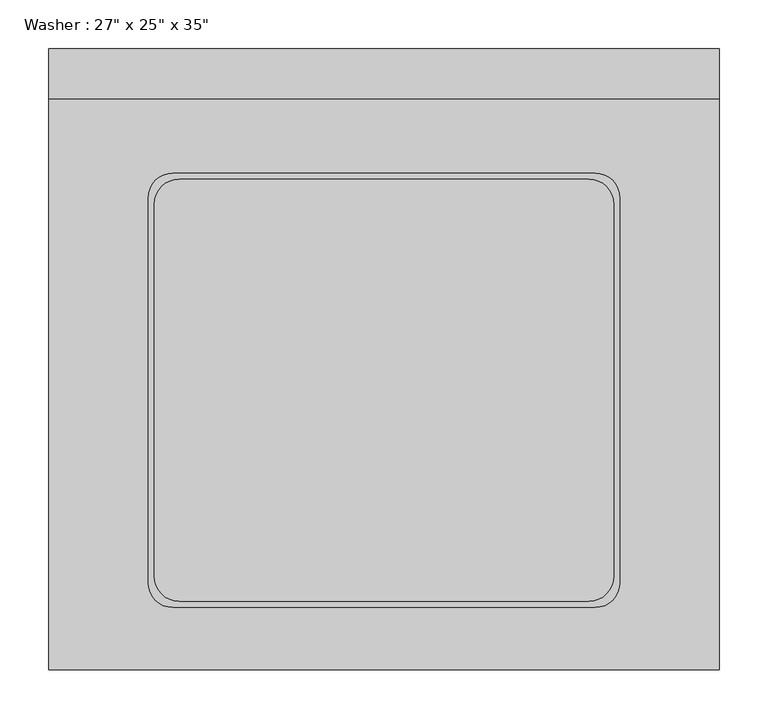
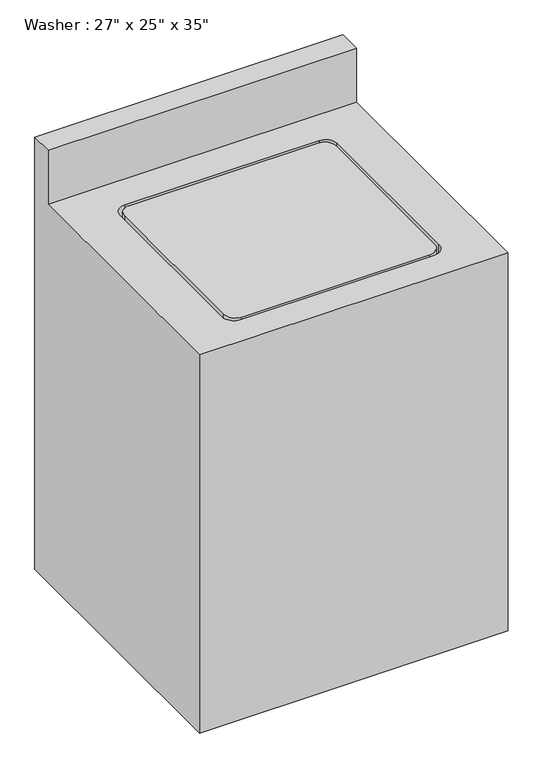
"""IFC4 building model written with IfcOpenShell, lengths in millimetres: proxy geometry."""

from ifc_helpers import new_model, si_unit, point, frame, frame_2d, origin, place, context, project, spatial, polyline, circle_curve, trimmed, segment, composite_curve, outline, extrude, source, transform, mapped, element, save
from ifc_brep_helpers import plane_surface, revolved_surface, advanced_brep


def proxy_e75280ca(model_context):
    return source(origin(), model_context, "Body", "SolidModel", [
        advanced_brep(
        [(77.5174685, 545.8495648, 889.0), (77.5174685, 545.8495648, 1016.0), (77.5174685, 596.6495648, 1016.0), (77.5174685, 596.6495648, 0.0), (77.5174685, -38.3504352, 0.0), (77.5174685, -38.3504352, 889.0), (763.3174685, 596.6495648, 1016.0), (763.3174685, 545.8495648, 1016.0), (763.3174685, 545.8495648, 889.0), (763.3174685, -38.3504352, 889.0), (763.3174685, -38.3504352, 0.0), (763.3174685, 596.6495648, 0.0), (204.5174685, 469.4681955, 889.0), (636.3174685, 469.4681955, 889.0), (661.7174685, 444.0681955, 889.0), (661.7174685, 50.5495648, 889.0), (636.3174685, 25.1495648, 889.0), (204.5174685, 25.1495648, 889.0), (179.1174685, 50.5495648, 889.0), (179.1174685, 444.0681955, 889.0), (636.3174685, 469.4681955, 838.2), (204.5174685, 469.4681955, 838.2), (179.1174685, 444.0681955, 838.2), (179.1174685, 50.5495648, 838.2), (204.5174685, 25.1495648, 838.2), (636.3174685, 25.1495648, 838.2), (661.7174685, 50.5495648, 838.2), (661.7174685, 444.0681955, 838.2)],
        [
            (0, 1),
            (1, 2),
            (2, 3),
            (3, 4),
            (4, 5),
            (5, 0),
            (6, 7),
            (7, 8),
            (8, 9),
            (9, 10),
            (10, 11),
            (11, 6),
            (0, 8),
            (7, 1),
            (6, 2),
            (11, 3),
            (5, 9),
            (12, 13),
            (13, 14, circle_curve(frame((636.3174685, 444.0681955, 889.0), z_axis=(0.0, 0.0, -1.0), x_axis=(0.0, -1.0, 0.0)), 25.4)),
            (14, 15),
            (15, 16, circle_curve(frame((636.3174685, 50.5495648, 889.0), z_axis=(0.0, 0.0, -1.0), x_axis=(0.0, -1.0, 0.0)), 25.4)),
            (16, 17),
            (17, 18, circle_curve(frame((204.5174685, 50.5495648, 889.0), z_axis=(0.0, 0.0, -1.0), x_axis=(0.0, -1.0, 0.0)), 25.4)),
            (18, 19),
            (19, 12, circle_curve(frame((204.5174685, 444.0681955, 889.0), z_axis=(0.0, 0.0, -1.0), x_axis=(0.0, -1.0, 0.0)), 25.4)),
            (10, 4),
            (20, 21),
            (21, 22, circle_curve(frame((204.5174685, 444.0681955, 838.2), z_axis=(0.0, 0.0, 1.0), x_axis=(0.0, -1.0, 0.0)), 25.4)),
            (22, 23),
            (23, 24, circle_curve(frame((204.5174685, 50.5495648, 838.2), z_axis=(0.0, 0.0, 1.0), x_axis=(0.0, -1.0, 0.0)), 25.4)),
            (24, 25),
            (25, 26, circle_curve(frame((636.3174685, 50.5495648, 838.2), z_axis=(0.0, 0.0, 1.0), x_axis=(0.0, -1.0, 0.0)), 25.4)),
            (26, 27),
            (27, 20, circle_curve(frame((636.3174685, 444.0681955, 838.2), z_axis=(0.0, 0.0, 1.0), x_axis=(0.0, -1.0, 0.0)), 25.4)),
            (20, 13),
            (12, 21),
            (19, 22),
            (18, 23),
            (17, 24),
            (16, 25),
            (15, 26),
            (14, 27),
        ],
        [
            plane_surface(frame((77.5174685, 545.8495648, 889.0), z_axis=(-1.0, 0.0, 0.0), x_axis=(0.0, 0.0, 1.0))),
            plane_surface(frame((763.3174685, 545.8495648, 889.0), z_axis=(1.0, 0.0, 0.0), x_axis=(0.0, 0.0, -1.0))),
            plane_surface(frame((77.5174685, 545.8495648, 889.0), z_axis=(0.0, -1.0, 0.0), x_axis=(1.0, 0.0, 0.0))),
            plane_surface(frame((77.5174685, 545.8495648, 1016.0), z_axis=(0.0, 0.0, 1.0), x_axis=(1.0, 0.0, 0.0))),
            plane_surface(frame((77.5174685, 596.6495648, 1016.0), z_axis=(0.0, 1.0, 0.0), x_axis=(1.0, 0.0, 0.0))),
            plane_surface(frame((77.5174685, -38.3504352, 889.0), z_axis=(0.0, 0.0, 1.0), x_axis=(0.0, -1.0, 0.0))),
            plane_surface(frame((77.5174685, -38.3504352, 0.0), z_axis=(0.0, 0.0, -1.0), x_axis=(0.0, 1.0, 0.0))),
            plane_surface(frame((77.5174685, -38.3504352, 889.0), z_axis=(0.0, -1.0, 0.0), x_axis=(0.0, 0.0, -1.0))),
            plane_surface(frame((204.5174685, 469.4681955, 838.2), z_axis=(0.0, 0.0, 1.0), x_axis=(1.0, 0.0, 0.0))),
            plane_surface(frame((636.3174685, 469.4681955, 889.0), z_axis=(0.0, -1.0, 0.0), x_axis=(0.0, 0.0, -1.0))),
            revolved_surface(polyline([(204.5174685, 418.6681955, 889.0), (204.5174685, 418.6681955, 838.2)]), (204.5174685, 444.0681955, 838.2), (0.0, 0.0, 1.0)),
            plane_surface(frame((179.1174685, 444.0681955, 889.0), z_axis=(1.0, 0.0, 0.0), x_axis=(0.0, 0.0, -1.0))),
            revolved_surface(polyline([(204.5174685, 25.1495648, 889.0), (204.5174685, 25.1495648, 838.2)]), (204.5174685, 50.5495648, 838.2), (0.0, 0.0, 1.0)),
            plane_surface(frame((204.5174685, 25.1495648, 889.0), z_axis=(0.0, 1.0, 0.0), x_axis=(0.0, 0.0, -1.0))),
            revolved_surface(polyline([(636.3174685, 25.1495648, 889.0), (636.3174685, 25.1495648, 838.2)]), (636.3174685, 50.5495648, 838.2), (0.0, 0.0, 1.0)),
            plane_surface(frame((661.7174685, 50.5495648, 889.0), z_axis=(-1.0, 0.0, 0.0), x_axis=(0.0, 0.0, -1.0))),
            revolved_surface(polyline([(636.3174685, 418.6681955, 889.0), (636.3174685, 418.6681955, 838.2)]), (636.3174685, 444.0681955, 838.2), (0.0, 0.0, 1.0)),
        ],
        [
            (0, [[1, 2, 3, 4, 5, 6]]),
            (1, [[7, 8, 9, 10, 11, 12]]),
            (2, [[-1, 13, -8, 14]]),
            (3, [[-2, -14, -7, 15]]),
            (4, [[-15, -12, 16, -3]]),
            (5, [[17, -9, -13, -6], [18, 19, 20, 21, 22, 23, 24, 25]]),
            (6, [[-16, -11, 26, -4]]),
            (7, [[-17, -5, -26, -10]]),
            (8, [[27, 28, 29, 30, 31, 32, 33, 34]]),
            (9, [[-27, 35, -18, 36]]),
            (10, [[-28, -36, -25, 37]]),
            (11, [[-29, -37, -24, 38]]),
            (12, [[-30, -38, -23, 39]]),
            (13, [[-31, -39, -22, 40]]),
            (14, [[-32, -40, -21, 41]]),
            (15, [[-33, -41, -20, 42]]),
            (16, [[-34, -42, -19, -35]]),
        ],
    ),
        extrude(outline(composite_curve([segment(trimmed(circle_curve(frame_2d((210.8674685, 437.8995648)), 25.4), [point((185.4674685, 437.8995648))], [point((210.8674685, 463.2995648))], False, "CARTESIAN"), True, "CONTINUOUS"), segment(polyline([(210.8674685, 463.2995648), (629.9674685, 463.2995648)]), True, "CONTINUOUS"), segment(trimmed(circle_curve(frame_2d((629.9674685, 437.8995648)), 25.4), [point((629.9674685, 463.2995648))], [point((655.3674685, 437.8995648))], False, "CARTESIAN"), True, "CONTINUOUS"), segment(polyline([(655.3674685, 437.8995648), (655.3674685, 56.8995648)]), True, "CONTINUOUS"), segment(trimmed(circle_curve(frame_2d((629.9674685, 56.8995648)), 25.4), [point((655.3674685, 56.8995648))], [point((629.9674685, 31.4995648))], False, "CARTESIAN"), True, "CONTINUOUS"), segment(polyline([(629.9674685, 31.4995648), (210.8674685, 31.4995648)]), True, "CONTINUOUS"), segment(trimmed(circle_curve(frame_2d((210.8674685, 56.8995648)), 25.4), [point((210.8674685, 31.4995648))], [point((185.4674685, 56.8995648))], False, "CARTESIAN"), True, "CONTINUOUS"), segment(polyline([(185.4674685, 56.8995648), (185.4674685, 437.8995648)]), True, "CONTINUOUS")], self_intersect=False)), frame((0.0, 0.0, 863.6), z_axis=(0.0, 0.0, 1.0), x_axis=(1.0, 0.0, 0.0)), (0.0, 0.0, 1.0), 25.4),
    ])


if __name__ == "__main__":
    model = new_model("IFC4")
    model_context = context("Model", 3, world=origin())
    ifc_project = project(units=[si_unit("LENGTHUNIT", "METRE", prefix="MILLI")], contexts=[model_context])
    site = spatial("IfcSite", under=ifc_project)
    building = spatial("IfcBuilding", under=site)
    placement = place(None, origin())
    proxy_shape = proxy_e75280ca(model_context)
    element("IfcBuildingElementProxy", 1, Name="Washer : 27\" x 25\" x 35\"", ObjectType="Washer : 27\" x 25\" x 35\"", at=placement, inside=building, context=model_context, shape_type="MappedRepresentation", body=[
        mapped(proxy_shape, transform((0.0, 0.0, 0.0), x_axis=(1.0, 0.0, 0.0), y_axis=(0.0, 1.0, 0.0), z_axis=(0.0, 0.0, 1.0))),
    ])
    save(model, "model.ifc")

# Revit data of these elements
# Type "Washer : 27\" x 25\" x 35\""
#   Label = "W"
#   Assembly Code = "E1090400"
#   Depth = 2' - 1"
#   Height = 2' - 11"
#   Width = 2' - 3"
#   Washer Material = Metal - Paint Finish - Ivory,Matte
#   Default Elevation = 0
# Element 1 (IfcBuildingElementProxy, "Washer : 27\" x 25\" x 35\"")
#   Materials on its faces: "Metal - Paint Finish - Ivory,Matte"
# Materials
#   "Metal - Paint Finish - Ivory,Matte": colour RGB 247 247 239, transparency 0
